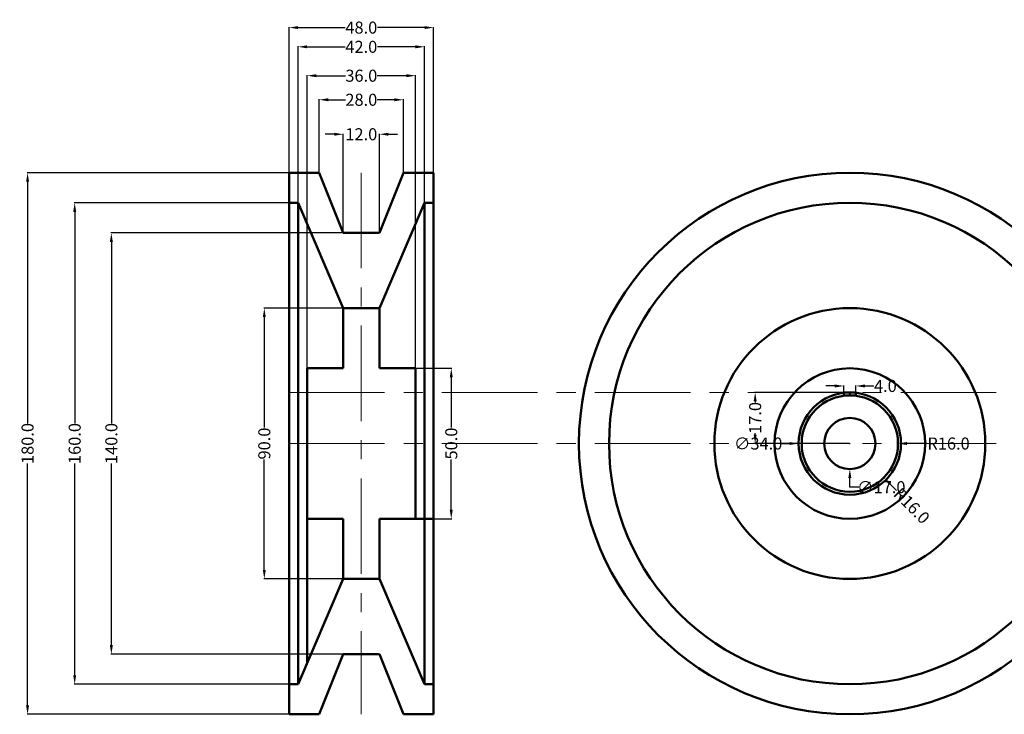
# Model space of a CAD drawing. Units: inches. Extents: x -30 to 602, y 452 to 930.
# Tile 1 of 3: x -30 to 297, y 452 to 683. Entities that reach past the tile are written whole.
import ezdxf

# ---------------------------------------------------------------- set-up
doc = ezdxf.new("R2010")
doc.units = ezdxf.units.IN
doc.header["$MEASUREMENT"] = 0
doc.linetypes.add('CENTER', pattern=[50.8, 31.75, -6.35, 6.35, -6.35])
for name, color, linetype, lineweight in [('M-CNTR', 1, 'CENTER', 18), ('M-DIMS', 2, 'Continuous', 25), ('M-OUTL', 7, 'Continuous', 50)]:
    doc.layers.add(name, color=color, linetype=linetype, lineweight=lineweight)
doc.styles.get("Standard").update_dxf_attribs({"font": 'arial.ttf'})
doc.dimstyles.get("Standard").update_dxf_attribs({"dimtxt": 4, "dimasz": 3, "dimexe": 0.18, "dimexo": 0.0625, "dimgap": 0.09, "dimtad": 0, "dimtoh": 1, "dimdec": 1, "dimzin": 0, "dimdsep": 46, "dimtxsty": 'Standard', "dimcen": 0.09, "dimadec": 0, "dimazin": 0, "dimtfac": 1, "dimtdec": 1, "dimtofl": 0, "dimtmove": 0, "dimatfit": 3, "dimfxl": 1, "dimtolj": 1, "dimtzin": 0, "dimarcsym": 0})

# ---------------------------------------------------------------- blocks, each defined once
blk = doc.blocks.new('*D31')
at = {"layer": 'Defpoints', "color": 0, "transparency": 16777216}
for p in [(59.17, 631.79), (-27.71, 451.79), (59.17, 451.79)]:
    blk.add_point(p, dxfattribs=at)
at = {"layer": 'M-DIMS', "color": 0, "lineweight": -2, "transparency": 16777216}
for p, q in [((59.11, 631.79), (-27.89, 631.79)), ((-27.71, 628.79), (-27.71, 548.43)), ((-27.71, 454.79), (-27.71, 535.15)), ((59.11, 451.79), (-27.89, 451.79))]:
    blk.add_line(p, q, dxfattribs=at)
at = {"layer": 'M-DIMS', "color": 0, "transparency": 16777216}
for points in [[(-28.21, 628.79), (-27.21, 628.79), (-27.71, 631.79)], [(-28.21, 454.79), (-27.21, 454.79), (-27.71, 451.79)]]:
    blk.add_solid(points, dxfattribs=at)
at = {"layer": 'M-DIMS', "color": 0, "transparency": 16777216, "insert": (-27.71, 541.79), "char_height": 4, "attachment_point": 5, "rotation": 90}
blk.add_mtext('\\A1;180.0', dxfattribs=at)
blk = doc.blocks.new('*D32')
at = {"layer": 'Defpoints', "color": 0, "transparency": 16777216}
for p in [(59.17, 621.79), (-12.06, 461.79), (59.17, 461.79)]:
    blk.add_point(p, dxfattribs=at)
at = {"layer": 'M-DIMS', "color": 0, "lineweight": -2, "transparency": 16777216}
for p, q in [((59.11, 621.79), (-12.24, 621.79)), ((-12.06, 618.79), (-12.06, 548.43)), ((-12.06, 464.79), (-12.06, 535.15)), ((59.11, 461.79), (-12.24, 461.79))]:
    blk.add_line(p, q, dxfattribs=at)
at = {"layer": 'M-DIMS', "color": 0, "transparency": 16777216}
for points in [[(-12.56, 618.79), (-11.56, 618.79), (-12.06, 621.79)], [(-12.56, 464.79), (-11.56, 464.79), (-12.06, 461.79)]]:
    blk.add_solid(points, dxfattribs=at)
at = {"layer": 'M-DIMS', "color": 0, "transparency": 16777216, "insert": (-12.06, 541.79), "char_height": 4, "attachment_point": 5, "rotation": 90}
blk.add_mtext('\\A1;160.0', dxfattribs=at)
blk = doc.blocks.new('*D33')
at = {"layer": 'Defpoints', "color": 0, "transparency": 16777216}
for p in [(77.17, 586.79), (50.94, 496.79), (77.17, 496.79)]:
    blk.add_point(p, dxfattribs=at)
at = {"layer": 'M-DIMS', "color": 0, "lineweight": -2, "transparency": 16777216}
for p, q in [((77.11, 586.79), (50.76, 586.79)), ((50.94, 583.79), (50.94, 547.07)), ((50.94, 499.79), (50.94, 536.51)), ((77.11, 496.79), (50.76, 496.79))]:
    blk.add_line(p, q, dxfattribs=at)
at = {"layer": 'M-DIMS', "color": 0, "transparency": 16777216}
for points in [[(50.44, 583.79), (51.44, 583.79), (50.94, 586.79)], [(50.44, 499.79), (51.44, 499.79), (50.94, 496.79)]]:
    blk.add_solid(points, dxfattribs=at)
at = {"layer": 'M-DIMS', "color": 0, "transparency": 16777216, "insert": (50.94, 541.79), "char_height": 4, "attachment_point": 5, "rotation": 90}
blk.add_mtext('\\A1;90.0', dxfattribs=at)
blk = doc.blocks.new('*D34')
at = {"layer": 'Defpoints', "color": 0, "transparency": 16777216}
for p in [(83.17, 611.79), (0.12, 471.79), (83.17, 471.79)]:
    blk.add_point(p, dxfattribs=at)
at = {"layer": 'M-DIMS', "color": 0, "lineweight": -2, "transparency": 16777216}
for p, q in [((83.11, 611.79), (-0.06, 611.79)), ((0.12, 608.79), (0.12, 548.43)), ((0.12, 474.79), (0.12, 535.15)), ((83.11, 471.79), (-0.06, 471.79))]:
    blk.add_line(p, q, dxfattribs=at)
at = {"layer": 'M-DIMS', "color": 0, "transparency": 16777216}
for points in [[(-0.38, 608.79), (0.62, 608.79), (0.12, 611.79)], [(-0.38, 474.79), (0.62, 474.79), (0.12, 471.79)]]:
    blk.add_solid(points, dxfattribs=at)
at = {"layer": 'M-DIMS', "color": 0, "transparency": 16777216, "insert": (0.12, 541.79), "char_height": 4, "attachment_point": 5, "rotation": 90}
blk.add_mtext('\\A1;140.0', dxfattribs=at)
blk = doc.blocks.new('*D35')
at = {"layer": 'Defpoints', "color": 0, "transparency": 16777216}
for p in [(107.17, 680.03), (59.17, 631.79), (107.17, 631.79)]:
    blk.add_point(p, dxfattribs=at)
at = {"layer": 'M-DIMS', "color": 0, "lineweight": -2, "transparency": 16777216}
for p, q in [((59.17, 631.85), (59.17, 680.21)), ((62.17, 680.03), (77.82, 680.03)), ((104.17, 680.03), (88.53, 680.03)), ((107.17, 631.85), (107.17, 680.21))]:
    blk.add_line(p, q, dxfattribs=at)
at = {"layer": 'M-DIMS', "color": 0, "transparency": 16777216}
for points in [[(62.17, 680.53), (62.17, 679.53), (59.17, 680.03)], [(104.17, 680.53), (104.17, 679.53), (107.17, 680.03)]]:
    blk.add_solid(points, dxfattribs=at)
at = {"layer": 'M-DIMS', "color": 0, "transparency": 16777216, "insert": (83.17, 680.03), "char_height": 4, "attachment_point": 5}
blk.add_mtext('\\A1;48.0', dxfattribs=at)
blk = doc.blocks.new('*D36')
at = {"layer": 'Defpoints', "color": 0, "transparency": 16777216}
for p in [(104.17, 673.64), (62.17, 621.79), (104.17, 621.79)]:
    blk.add_point(p, dxfattribs=at)
at = {"layer": 'M-DIMS', "color": 0, "lineweight": -2, "transparency": 16777216}
for p, q in [((62.17, 621.85), (62.17, 673.82)), ((65.17, 673.64), (77.82, 673.64)), ((101.17, 673.64), (88.53, 673.64)), ((104.17, 621.85), (104.17, 673.82))]:
    blk.add_line(p, q, dxfattribs=at)
at = {"layer": 'M-DIMS', "color": 0, "transparency": 16777216}
for points in [[(65.17, 674.14), (65.17, 673.14), (62.17, 673.64)], [(101.17, 674.14), (101.17, 673.14), (104.17, 673.64)]]:
    blk.add_solid(points, dxfattribs=at)
at = {"layer": 'M-DIMS', "color": 0, "transparency": 16777216, "insert": (83.17, 673.64), "char_height": 4, "attachment_point": 5}
blk.add_mtext('\\A1;42.0', dxfattribs=at)
blk = doc.blocks.new('*D37')
at = {"layer": 'Defpoints', "color": 0, "transparency": 16777216}
for p in [(101.17, 664.04), (65.17, 566.79), (101.17, 566.79)]:
    blk.add_point(p, dxfattribs=at)
at = {"layer": 'M-DIMS', "color": 0, "lineweight": -2, "transparency": 16777216}
for p, q in [((65.17, 566.85), (65.17, 664.22)), ((101.17, 566.85), (101.17, 664.22)), ((68.17, 664.04), (77.9, 664.04)), ((98.17, 664.04), (88.45, 664.04))]:
    blk.add_line(p, q, dxfattribs=at)
at = {"layer": 'M-DIMS', "color": 0, "transparency": 16777216}
for points in [[(68.17, 664.54), (68.17, 663.54), (65.17, 664.04)], [(98.17, 664.54), (98.17, 663.54), (101.17, 664.04)]]:
    blk.add_solid(points, dxfattribs=at)
at = {"layer": 'M-DIMS', "color": 0, "transparency": 16777216, "insert": (83.17, 664.04), "char_height": 4, "attachment_point": 5}
blk.add_mtext('\\A1;36.0', dxfattribs=at)
blk = doc.blocks.new('*D38')
at = {"layer": 'Defpoints', "color": 0, "transparency": 16777216}
for p in [(97.17, 656.04), (69.17, 631.79), (97.17, 631.79)]:
    blk.add_point(p, dxfattribs=at)
at = {"layer": 'M-DIMS', "color": 0, "lineweight": -2, "transparency": 16777216}
for p, q in [((69.17, 631.85), (69.17, 656.22)), ((72.17, 656.04), (77.86, 656.04)), ((94.17, 656.04), (88.49, 656.04)), ((97.17, 631.85), (97.17, 656.22))]:
    blk.add_line(p, q, dxfattribs=at)
at = {"layer": 'M-DIMS', "color": 0, "transparency": 16777216}
for points in [[(72.17, 656.54), (72.17, 655.54), (69.17, 656.04)], [(94.17, 656.54), (94.17, 655.54), (97.17, 656.04)]]:
    blk.add_solid(points, dxfattribs=at)
at = {"layer": 'M-DIMS', "color": 0, "transparency": 16777216, "insert": (83.17, 656.04), "char_height": 4, "attachment_point": 5}
blk.add_mtext('\\A1;28.0', dxfattribs=at)
blk = doc.blocks.new('*D39')
at = {"layer": 'Defpoints', "color": 0, "transparency": 16777216}
for p in [(89.17, 644.58), (77.17, 611.79), (89.17, 611.79)]:
    blk.add_point(p, dxfattribs=at)
at = {"layer": 'M-DIMS', "color": 0, "lineweight": -2, "transparency": 16777216}
for p, q in [((74.17, 644.58), (71.17, 644.58)), ((77.17, 611.85), (77.17, 644.76)), ((89.17, 611.85), (89.17, 644.76)), ((92.17, 644.58), (95.17, 644.58))]:
    blk.add_line(p, q, dxfattribs=at)
at = {"layer": 'M-DIMS', "color": 0, "transparency": 16777216}
for points in [[(74.17, 645.08), (74.17, 644.08), (77.17, 644.58)], [(92.17, 645.08), (92.17, 644.08), (89.17, 644.58)]]:
    blk.add_solid(points, dxfattribs=at)
at = {"layer": 'M-DIMS', "color": 0, "transparency": 16777216, "insert": (83.17, 644.58), "char_height": 4, "attachment_point": 5}
blk.add_mtext('\\A1;12.0', dxfattribs=at)
blk = doc.blocks.new('*D40')
at = {"layer": 'Defpoints', "color": 0, "transparency": 16777216}
for p in [(101.17, 566.79), (101.17, 516.79), (113.05, 516.79)]:
    blk.add_point(p, dxfattribs=at)
at = {"layer": 'M-DIMS', "color": 0, "lineweight": -2, "transparency": 16777216}
for p, q in [((101.24, 566.79), (113.23, 566.79)), ((113.05, 563.79), (113.05, 547.07)), ((113.05, 519.79), (113.05, 536.51)), ((101.24, 516.79), (113.23, 516.79))]:
    blk.add_line(p, q, dxfattribs=at)
at = {"layer": 'M-DIMS', "color": 0, "transparency": 16777216}
for points in [[(112.55, 563.79), (113.55, 563.79), (113.05, 566.79)], [(112.55, 519.79), (113.55, 519.79), (113.05, 516.79)]]:
    blk.add_solid(points, dxfattribs=at)
at = {"layer": 'M-DIMS', "color": 0, "transparency": 16777216, "insert": (113.05, 541.79), "char_height": 4, "attachment_point": 5, "rotation": 90}
blk.add_mtext('\\A1;50.0', dxfattribs=at)
blk = doc.blocks.new('*D41')
at = {"layer": 'Defpoints', "color": 0, "transparency": 16777216}
for p in [(245.47, 558.79), (214.02, 541.79), (245.47, 541.79)]:
    blk.add_point(p, dxfattribs=at)
at = {"layer": 'M-DIMS', "color": 0, "lineweight": -2, "transparency": 16777216}
for p, q in [((245.41, 558.79), (213.84, 558.79)), ((214.02, 555.79), (214.02, 555.38)), ((214.02, 544.79), (214.02, 545.2)), ((245.41, 541.79), (213.84, 541.79))]:
    blk.add_line(p, q, dxfattribs=at)
at = {"layer": 'M-DIMS', "color": 0, "transparency": 16777216}
for points in [[(213.52, 555.79), (214.52, 555.79), (214.02, 558.79)], [(213.52, 544.79), (214.52, 544.79), (214.02, 541.79)]]:
    blk.add_solid(points, dxfattribs=at)
at = {"layer": 'M-DIMS', "color": 0, "transparency": 16777216, "insert": (214.02, 550.29), "char_height": 4, "attachment_point": 5, "rotation": 90}
blk.add_mtext('\\A1;17.0', dxfattribs=at)
blk = doc.blocks.new('*D42')
at = {"layer": 'Defpoints', "color": 0, "transparency": 16777216}
for p in [(247.47, 560.92), (243.47, 558.23), (247.47, 558.23)]:
    blk.add_point(p, dxfattribs=at)
at = {"layer": 'M-DIMS', "color": 0, "lineweight": -2, "transparency": 16777216}
for p, q in [((240.47, 560.92), (237.47, 560.92)), ((243.47, 558.29), (243.47, 561.1)), ((247.47, 558.29), (247.47, 561.1)), ((250.47, 560.92), (253.47, 560.92))]:
    blk.add_line(p, q, dxfattribs=at)
at = {"layer": 'M-DIMS', "color": 0, "transparency": 16777216}
for points in [[(240.47, 561.42), (240.47, 560.42), (243.47, 560.92)], [(250.47, 561.42), (250.47, 560.42), (247.47, 560.92)]]:
    blk.add_solid(points, dxfattribs=at)
at = {"layer": 'M-DIMS', "color": 0, "transparency": 16777216, "insert": (257.28, 560.92), "char_height": 4, "attachment_point": 5}
blk.add_mtext('\\A1;4.0', dxfattribs=at)
blk = doc.blocks.new('*D43')
at = {"layer": 'Defpoints', "color": 0, "transparency": 16777216}
for p in [(245.47, 541.79), (256.75, 530.44)]:
    blk.add_point(p, dxfattribs=at)
at = {"layer": 'M-DIMS', "color": 0, "lineweight": -2, "transparency": 16777216}
for p, q in [((245.38, 541.79), (245.56, 541.79)), ((245.47, 541.7), (245.47, 541.88)), ((260.98, 526.19), (258.87, 528.32))]:
    blk.add_line(p, q, dxfattribs=at)
at = {"layer": 'M-DIMS', "color": 0, "transparency": 16777216}
blk.add_solid([(259.22, 528.67), (258.51, 527.96), (256.75, 530.44)], dxfattribs=at)
at = {"layer": 'M-DIMS', "color": 0, "transparency": 16777216, "insert": (266.05, 521.09), "char_height": 4, "attachment_point": 5, "rotation": 314.8337}
blk.add_mtext('\\A1;R16.0', dxfattribs=at)
blk = doc.blocks.new('*D65')
at = {"layer": 'Defpoints', "color": 0, "transparency": 16777216}
for p in [(245.47, 550.29), (245.47, 533.29)]:
    blk.add_point(p, dxfattribs=at)
at = {"layer": 'M-DIMS', "color": 0, "lineweight": -2, "transparency": 16777216}
for p, q in [((245.38, 541.79), (245.56, 541.79)), ((245.47, 541.7), (245.47, 541.88)), ((245.47, 527.29), (245.47, 530.29)), ((248.47, 527.29), (245.47, 527.29))]:
    blk.add_line(p, q, dxfattribs=at)
at = {"layer": 'M-DIMS', "color": 0, "transparency": 16777216}
blk.add_solid([(245.97, 530.29), (244.97, 530.29), (245.47, 533.29)], dxfattribs=at)
at = {"layer": 'M-DIMS', "color": 0, "transparency": 16777216, "insert": (255.93, 527.29), "char_height": 4, "attachment_point": 5}
blk.add_mtext('\\A1;∅17.0', dxfattribs=at)
blk = doc.blocks.new('*D66')
at = {"layer": 'Defpoints', "color": 0, "transparency": 16777216}
for p in [(245.47, 541.79), (261.47, 541.79)]:
    blk.add_point(p, dxfattribs=at)
at = {"layer": 'M-DIMS', "color": 0, "lineweight": -2, "transparency": 16777216}
for p, q in [((245.38, 541.79), (245.56, 541.79)), ((245.47, 541.7), (245.47, 541.88)), ((271.07, 541.79), (264.47, 541.79))]:
    blk.add_line(p, q, dxfattribs=at)
at = {"layer": 'M-DIMS', "color": 0, "transparency": 16777216}
blk.add_solid([(264.47, 542.29), (264.47, 541.29), (261.47, 541.79)], dxfattribs=at)
at = {"layer": 'M-DIMS', "color": 0, "transparency": 16777216, "insert": (278.27, 541.79), "char_height": 4, "attachment_point": 5}
blk.add_mtext('\\A1;R16.0', dxfattribs=at)
blk = doc.blocks.new('*D67')
at = {"layer": 'Defpoints', "color": 0, "transparency": 16777216}
for p in [(228.47, 541.79), (262.47, 541.79)]:
    blk.add_point(p, dxfattribs=at)
at = {"layer": 'M-DIMS', "color": 0, "lineweight": -2, "transparency": 16777216}
for p, q in [((222.47, 541.79), (225.47, 541.79)), ((245.38, 541.79), (245.56, 541.79)), ((245.47, 541.7), (245.47, 541.88))]:
    blk.add_line(p, q, dxfattribs=at)
at = {"layer": 'M-DIMS', "color": 0, "transparency": 16777216}
blk.add_solid([(225.47, 542.29), (225.47, 541.29), (228.47, 541.79)], dxfattribs=at)
at = {"layer": 'M-DIMS', "color": 0, "transparency": 16777216, "insert": (215.02, 541.79), "char_height": 4, "attachment_point": 5}
blk.add_mtext('\\A1;∅34.0', dxfattribs=at)

msp = doc.modelspace()

# ---------------------------------------------------------------- linework, layer by layer
at = {"layer": 'M-CNTR'}
for p, q in [((83.17, 631.79), (83.17, 451.79)), ((59.17, 558.79), (462.28, 558.79)), ((59.17, 541.79), (462.28, 541.79))]:
    msp.add_line(p, q, dxfattribs=at)
at = {"layer": 'M-OUTL'}
for p, q in [((59.17, 631.79), (69.17, 631.79)), ((59.17, 451.79), (59.17, 631.79)), ((77.17, 611.79), (69.17, 631.79)), ((89.17, 611.79), (97.17, 631.79)), ((97.17, 631.79), (107.17, 631.79)), ((107.17, 631.79), (107.17, 451.79)), ((59.17, 621.79), (62.17, 621.79)), ((62.17, 461.79), (62.17, 621.79)), ((77.17, 586.79), (62.17, 621.79)), ((89.17, 586.79), (104.17, 621.79)), ((104.17, 621.79), (104.17, 461.79)), ((104.17, 621.79), (107.17, 621.79)), ((77.17, 611.79), (89.17, 611.79)), ((77.17, 586.79), (89.17, 586.79)), ((77.17, 586.79), (77.17, 566.79)), ((89.17, 586.79), (89.17, 566.79)), ((65.17, 566.79), (65.17, 468.79)), ((65.17, 566.79), (77.17, 566.79)), ((89.17, 566.79), (101.17, 566.79)), ((101.17, 566.79), (101.17, 516.79)), ((243.47, 557.67), (243.47, 558.79)), ((243.47, 558.79), (247.47, 558.79)), ((245.47, 557.79), (245.47, 558.79)), ((247.47, 557.67), (247.47, 558.79)), ((65.17, 516.79), (77.17, 516.79)), ((77.17, 496.79), (77.17, 516.79)), ((89.17, 496.79), (89.17, 516.79)), ((89.17, 516.79), (107.17, 516.79)), ((77.17, 496.79), (62.17, 461.79)), ((77.17, 496.79), (89.17, 496.79)), ((89.17, 496.79), (104.17, 461.79)), ((69.17, 451.79), (77.17, 471.79)), ((77.17, 471.79), (89.17, 471.79)), ((97.17, 451.79), (89.17, 471.79)), ((59.17, 461.79), (62.17, 461.79)), ((104.17, 461.79), (107.17, 461.79)), ((69.17, 451.79), (59.17, 451.79)), ((107.17, 451.79), (97.17, 451.79))]:
    msp.add_line(p, q, dxfattribs=at)
for radius in [90, 80, 45, 25, 17, 16, 8.5]:
    msp.add_circle((245.47, 541.79), radius, dxfattribs=at)

# ---------------------------------------------------------------- dimensions: what is measured, and where the dimension line sits
at = {"layer": 'M-DIMS'}
for base, p1, p2, picture, middle in [((107.17, 680.03), (59.17, 631.79), (107.17, 631.79), '*D35', (83.17, 680.03)), ((104.17, 673.64), (62.17, 621.79), (104.17, 621.79), '*D36', (83.17, 673.64)), ((101.17, 664.04), (65.17, 566.79), (101.17, 566.79), '*D37', (83.17, 664.04)), ((97.17, 656.04), (69.17, 631.79), (97.17, 631.79), '*D38', (83.17, 656.04)), ((89.17, 644.58), (77.17, 611.79), (89.17, 611.79), '*D39', (83.17, 644.58)), ((247.47, 560.92), (243.47, 558.23), (247.47, 558.23), '*D42', (257.28, 560.92))]:
    dim = msp.add_linear_dim(base=base, p1=p1, p2=p2, dimstyle='Standard', override={"dimclrd": 0, "dimclre": 0, "dimclrt": 0}, dxfattribs=at)
    dim.commit()
    dim.dimension.update_dxf_attribs({"geometry": picture, "text_midpoint": middle})
for base, p1, p2, picture, middle in [((-27.71, 451.79), (59.17, 631.79), (59.17, 451.79), '*D31', (-27.71, 541.79)), ((-12.06, 461.79), (59.17, 621.79), (59.17, 461.79), '*D32', (-12.06, 541.79)), ((0.12, 471.79), (83.17, 611.79), (83.17, 471.79), '*D34', (0.12, 541.79)), ((50.94, 496.79), (77.17, 586.79), (77.17, 496.79), '*D33', (50.94, 541.79)), ((113.05, 516.79), (101.17, 566.79), (101.17, 516.79), '*D40', (113.05, 541.79)), ((214.02, 541.79), (245.47, 558.79), (245.47, 541.79), '*D41', (214.02, 550.29))]:
    dim = msp.add_linear_dim(base=base, p1=p1, p2=p2, angle=90, dimstyle='Standard', override={"dimclrd": 0, "dimclre": 0, "dimclrt": 0}, dxfattribs=at)
    dim.commit()
    dim.dimension.update_dxf_attribs({"geometry": picture, "text_midpoint": middle})
for p1, p2, picture, middle in [((245.47, 550.29), (245.47, 533.29), '*D65', (255.93, 527.29)), ((262.47, 541.79), (228.47, 541.79), '*D67', (215.02, 541.79))]:
    dim = msp.add_diameter_dim_2p(p1=p1, p2=p2, dimstyle='Standard', override={"dimdec": 1, "dimlfac": 1, "dimrnd": 0, "dimzin": 0, "dimdsep": 46, "dimlunit": 2}, dxfattribs=at)
    dim.commit()
    dim.dimension.update_dxf_attribs({"geometry": picture, "text_midpoint": middle})
dim = msp.add_radius_dim(center=(245.47, 541.79), mpoint=(261.47, 541.79), dimstyle='Standard', override={"dimdec": 1, "dimlfac": 1, "dimrnd": 0, "dimzin": 0, "dimdsep": 46, "dimlunit": 2}, dxfattribs=at)
dim.commit()
dim.dimension.update_dxf_attribs({"geometry": '*D66', "text_midpoint": (271.07, 541.79), "dimtype": 164})
dim = msp.add_radius_dim(center=(245.47, 541.79), mpoint=(256.75, 530.44), dimstyle='Standard', override={"dimclrd": 0, "dimclre": 0, "dimclrt": 0}, dxfattribs=at)
dim.commit()
dim.dimension.update_dxf_attribs({"geometry": '*D43', "text_midpoint": (266.05, 521.09)})

doc.saveas('drawing.dxf')
